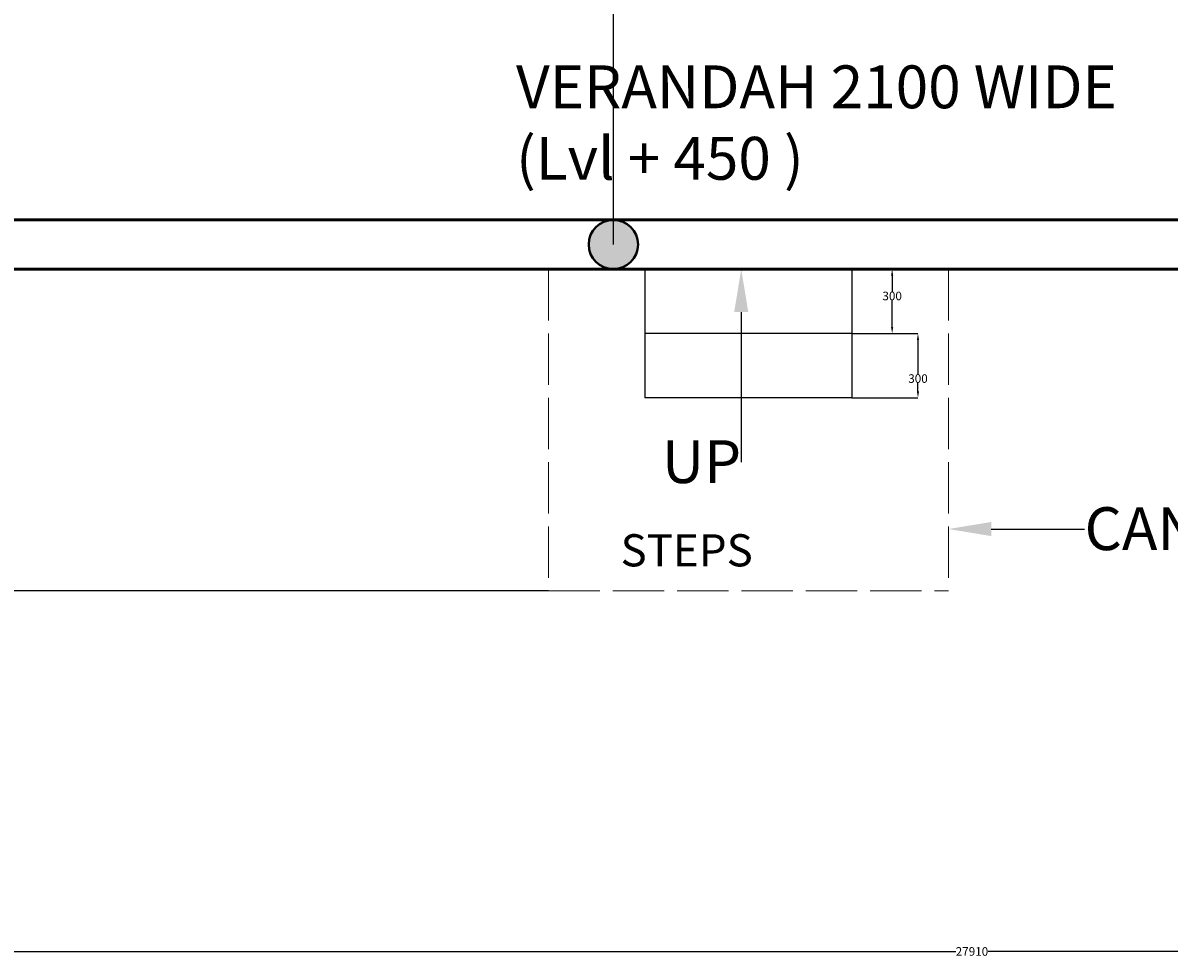
# Model space of a CAD drawing. Units: millimetres. Extents: x -17156 to 39375, y -45872 to -24892.
# Tile 4 of 12: x -5337 to 7, y -45872 to -41514. Entities that reach past the tile are written whole.
import ezdxf
from ezdxf import colors
from ezdxf.entities.mleader import LeaderData, LeaderLine
from ezdxf.math import Vec2, Vec3

# ---------------------------------------------------------------- set-up
doc = ezdxf.new("R2010")
doc.units = ezdxf.units.MM
doc.header["$MEASUREMENT"] = 0
doc.linetypes.add('ACAD_ISO02W100', pattern=[15, 12, -3])
for name, color, linetype, lineweight in [('A-ANNO-DIMS', 2, 'Continuous', 18), ('A-ANNO-TEXT', 4, 'Continuous', 18), ('A-AREA-IDEN', 4, 'Continuous', 25), ('A-COLS', 7, 'Continuous', 40), ('A-ROOF-OVHD', 8, 'ACAD_ISO02W100', 18), ('STEPS', 2, 'Continuous', 25), ('WALLS', 5, 'Continuous', 50)]:
    doc.layers.add(name, color=color, linetype=linetype, lineweight=lineweight)
doc.layers.add('A-COLS-PATT', color=114, linetype='Continuous', lineweight=13, true_color=0x139b48)
doc.styles.get("Standard").update_dxf_attribs({"font": 'arial.ttf'})
doc.dimstyles.get("Standard").update_dxf_attribs({"dimtxt": 40, "dimasz": 30.18, "dimexe": 0, "dimexo": 0.0625, "dimgap": 0.09, "dimtad": 0, "dimtih": 1, "dimtoh": 1, "dimdec": 0, "dimzin": 0, "dimdsep": 46, "dimtxsty": 'Standard', "dimcen": 0.09, "dimadec": 0, "dimazin": 0, "dimtfac": 1, "dimtdec": 0, "dimtofl": 0, "dimtmove": 0, "dimatfit": 3, "dimfxl": 1, "dimtolj": 1, "dimtzin": 0, "dimarcsym": 0})

# ---------------------------------------------------------------- blocks, each defined once
blk = doc.blocks.new('*D98')
at = {"layer": 'A-ANNO-DIMS', "color": 0, "lineweight": -2, "transparency": 16777216}
for p, q in [((-1472.3, -42962.8), (-1163.9, -42962.8)), ((-1163.9, -42993), (-1163.9, -43152.7)), ((-1163.9, -43232.7), (-1163.9, -43193.7)), ((-1472.3, -43262.8), (-1163.9, -43262.8))]:
    blk.add_line(p, q, dxfattribs=at)
at = {"layer": 'A-ANNO-DIMS', "color": 0, "lineweight": 100, "transparency": 16777216}
for points in [[(-1169, -42993), (-1158.9, -42993), (-1163.9, -42962.8)], [(-1169, -43232.7), (-1158.9, -43232.7), (-1163.9, -43262.8)]]:
    blk.add_solid(points, dxfattribs=at)
at = {"layer": 'Defpoints', "color": 0, "lineweight": 100, "transparency": 16777216}
for p in [(-1472.3, -42962.8), (-1163.9, -42962.8), (-1472.3, -43262.8)]:
    blk.add_point(p, dxfattribs=at)
at = {"layer": 'A-ANNO-DIMS', "color": 0, "transparency": 16777216, "insert": (-1163.9, -43173.2), "char_height": 40, "attachment_point": 5}
blk.add_mtext('\\A1;300', dxfattribs=at)
blk = doc.blocks.new('*D99')
at = {"layer": 'A-ANNO-DIMS', "color": 0, "lineweight": -2, "transparency": 16777216}
for p, q in [((-1472.3, -42662.8), (-1284.4, -42662.8)), ((-1284.4, -42693), (-1284.4, -42767.4)), ((-1284.4, -42932.7), (-1284.4, -42808.4)), ((-1472.3, -42962.8), (-1284.4, -42962.8))]:
    blk.add_line(p, q, dxfattribs=at)
at = {"layer": 'A-ANNO-DIMS', "color": 0, "lineweight": 100, "transparency": 16777216}
for points in [[(-1289.4, -42693), (-1279.4, -42693), (-1284.4, -42662.8)], [(-1289.4, -42932.7), (-1279.4, -42932.7), (-1284.4, -42962.8)]]:
    blk.add_solid(points, dxfattribs=at)
at = {"layer": 'Defpoints', "color": 0, "lineweight": 100, "transparency": 16777216}
for p in [(-1472.3, -42662.8), (-1284.4, -42662.8), (-1472.3, -42962.8)]:
    blk.add_point(p, dxfattribs=at)
at = {"layer": 'A-ANNO-DIMS', "color": 0, "transparency": 16777216, "insert": (-1284.4, -42787.9), "char_height": 40, "attachment_point": 5}
blk.add_mtext('\\A1;300', dxfattribs=at)
blk = doc.blocks.new('*D145')
at = {"layer": 'A-ANNO-DIMS', "color": 0, "lineweight": -2, "transparency": 16777216}
for p, q in [((-6237.4, -27247.8), (-17080.3, -27247.8)), ((-17080.3, -27278), (-17080.3, -35684.8)), ((-17080.3, -44132.7), (-17080.3, -35725.9)), ((-2887.4, -44162.8), (-17080.3, -44162.8))]:
    blk.add_line(p, q, dxfattribs=at)
at = {"layer": 'A-ANNO-DIMS', "color": 0, "lineweight": 100, "transparency": 16777216}
for points in [[(-17085.4, -27278), (-17075.3, -27278), (-17080.3, -27247.8)], [(-17085.4, -44132.7), (-17075.3, -44132.7), (-17080.3, -44162.8)]]:
    blk.add_solid(points, dxfattribs=at)
at = {"layer": 'Defpoints', "color": 0, "lineweight": 100, "transparency": 16777216}
for p in [(-6237.3, -27247.8), (-17080.3, -44162.8), (-2887.3, -44162.8)]:
    blk.add_point(p, dxfattribs=at)
at = {"layer": 'A-ANNO-DIMS', "color": 0, "transparency": 16777216, "insert": (-17080.3, -35705.3), "char_height": 40, "attachment_point": 5}
blk.add_mtext('\\A1;16915', dxfattribs=at)
blk = doc.blocks.new('*D146')
at = {"layer": 'A-ANNO-DIMS', "color": 0, "lineweight": -2, "transparency": 16777216}
for p, q in [((-14867.3, -42732.9), (-14867.3, -45845.8)), ((13042.7, -42732.9), (13042.7, -45845.8)), ((-14837.2, -45845.8), (-988, -45845.8)), ((13012.5, -45845.8), (-836.7, -45845.8))]:
    blk.add_line(p, q, dxfattribs=at)
at = {"layer": 'A-ANNO-DIMS', "color": 0, "lineweight": 100, "transparency": 16777216}
for points in [[(-14837.2, -45840.8), (-14837.2, -45850.9), (-14867.3, -45845.8)], [(13012.5, -45840.8), (13012.5, -45850.9), (13042.7, -45845.8)]]:
    blk.add_solid(points, dxfattribs=at)
at = {"layer": 'Defpoints', "color": 0, "lineweight": 100, "transparency": 16777216}
for p in [(-14867.3, -42732.8), (13042.7, -42732.8), (13042.7, -45845.8)]:
    blk.add_point(p, dxfattribs=at)
at = {"layer": 'A-ANNO-DIMS', "color": 0, "transparency": 16777216, "insert": (-912.3, -45845.8), "char_height": 40, "attachment_point": 5}
blk.add_mtext('\\A1;27910', dxfattribs=at)
blk = doc.blocks.new('*D151')
at = {"layer": 'A-ANNO-DIMS', "color": 0, "lineweight": -2, "transparency": 16777216}
for p, q in [((-6122.3, -42547.8), (-6122.3, -25564.8)), ((-6092.2, -25564.8), (-4413.2, -25564.8)), ((-2614.5, -25564.8), (-4293.5, -25564.8)), ((-2584.3, -42547.8), (-2584.3, -25564.8))]:
    blk.add_line(p, q, dxfattribs=at)
at = {"layer": 'A-ANNO-DIMS', "color": 0, "lineweight": 100, "transparency": 16777216}
for points in [[(-6092.2, -25559.8), (-6092.2, -25569.9), (-6122.3, -25564.8)], [(-2614.5, -25559.8), (-2614.5, -25569.9), (-2584.3, -25564.8)]]:
    blk.add_solid(points, dxfattribs=at)
at = {"layer": 'Defpoints', "color": 0, "lineweight": 100, "transparency": 16777216}
for p in [(-2584.3, -25564.8), (-6122.3, -42547.8), (-2584.3, -42547.8)]:
    blk.add_point(p, dxfattribs=at)
at = {"layer": 'A-ANNO-DIMS', "color": 0, "transparency": 16777216, "insert": (-4353.3, -25564.8), "char_height": 40, "attachment_point": 5}
blk.add_mtext('\\A1;3538', dxfattribs=at)

msp = doc.modelspace()

# ---------------------------------------------------------------- hatches: boundary and pattern name
at = {"layer": 'A-COLS-PATT'}
h = msp.add_hatch(color=256, dxfattribs=at)
h.dxf.hatch_style = 1
h.paths.add_polyline_path([(-6007.35, -42547.85, 1), (-6237.35, -42547.85, 1)])
h.paths.add_polyline_path([(-2699.35, -42547.85, 1), (-2469.35, -42547.85, 1)])
h.paths.add_polyline_path([(424.65, -42547.85, 1), (654.65, -42547.85, 1)])
h.paths.add_polyline_path([(3997.65, -42547.85, 1), (4227.65, -42547.85, 1)])
h.paths.add_polyline_path([(1581.84, -34499.85), (1481.84, -34499.85), (1481.84, -34599.85), (1581.84, -34599.85)])
h.paths.add_polyline_path([(3181.84, -34499.85), (3081.84, -34499.85), (3081.84, -34599.85), (3181.84, -34599.85)])
h.paths.add_polyline_path([(-162.32, -34499.85), (-262.32, -34499.85), (-262.32, -34599.85), (-162.32, -34599.85)])
h.paths.add_polyline_path([(-1762.32, -34499.85), (-1862.32, -34499.85), (-1862.32, -34599.85), (-1762.32, -34599.85)])
h.paths.add_polyline_path([(-3445.85, -34499.85), (-3545.85, -34499.85), (-3545.85, -34599.85), (-3445.85, -34599.85)])
h.paths.add_polyline_path([(-5045.85, -34499.85), (-5145.85, -34499.85), (-5145.85, -34599.85), (-5045.85, -34599.85)])

# ---------------------------------------------------------------- linework, layer by layer
at = {"layer": 'A-COLS'}
msp.add_circle((-2584.35, -42547.85), 115, dxfattribs=at)
at = {"layer": 'A-ROOF-OVHD', "ltscale": 20}
for p, q in [((-2887.35, -42662.85), (-2887.35, -44162.85)), ((-1022.35, -42662.85), (-1022.35, -44162.85)), ((-2887.35, -44162.85), (-1022.35, -44162.85))]:
    msp.add_line(p, q, dxfattribs=at)
at = {"layer": 'STEPS'}
for p, q in [((-2437.35, -42662.85), (-2437.35, -43262.85)), ((-1472.35, -42662.85), (-1472.35, -43262.85)), ((-1472.35, -42962.85), (-2437.35, -42962.85)), ((-1472.35, -43262.85), (-2437.35, -43262.85))]:
    msp.add_line(p, q, dxfattribs=at)
at = {"layer": 'WALLS'}
for p, q in [((12592.65, -42432.85), (-10997.35, -42432.85)), ((12822.65, -42662.85), (-14797.35, -42662.85))]:
    msp.add_line(p, q, dxfattribs=at)

# ---------------------------------------------------------------- texts
at = {"layer": 'A-ANNO-TEXT', "insert": (-2550.74, -43899.35), "char_height": 150, "attachment_point": 1}
msp.add_mtext_dynamic_manual_height_columns('{STEPS}', width=605.9062, gutter_width=1, heights=[0], dxfattribs=at)
at = {"layer": 'A-AREA-IDEN', "insert": (-3038.04, -41712.25), "char_height": 200, "attachment_point": 1}
msp.add_mtext_dynamic_manual_height_columns('{VERANDAH 2100 WIDE\\P(Lvl + 450 )}', width=5045.4894, gutter_width=1, heights=[0], dxfattribs=at)

# ---------------------------------------------------------------- dimensions: what is measured, and where the dimension line sits
at = {"layer": 'A-ANNO-DIMS'}
for base, p1, p2, picture, middle in [((-2584.35, -25564.85), (-6122.35, -42547.85), (-2584.35, -42547.85), '*D151', (-4353.35, -25564.85)), ((13042.65, -45845.85), (-14867.35, -42732.85), (13042.65, -42732.85), '*D146', (-912.35, -45845.85))]:
    dim = msp.add_linear_dim(base=base, p1=p1, p2=p2, dimstyle='Standard', override={"dimdec": 0, "dimlfac": 1, "dimrnd": 0, "dimzin": 0, "dimdsep": 46, "dimlunit": 2}, dxfattribs=at)
    dim.commit()
    dim.dimension.update_dxf_attribs({"geometry": picture, "text_midpoint": middle})
dim = msp.add_linear_dim(base=(-17080.35, -44162.85), p1=(-6237.35, -27247.85), p2=(-2887.35, -44162.85), angle=90, dimstyle='Standard', override={"dimdec": 0, "dimlfac": 1, "dimrnd": 0, "dimzin": 0, "dimdsep": 46, "dimlunit": 2}, dxfattribs=at)
dim.commit()
dim.dimension.update_dxf_attribs({"geometry": '*D145', "text_midpoint": (-17080.35, -35705.35)})
for base, p1, p2, picture, middle in [((-1284.39, -42662.85), (-1472.35, -42962.85), (-1472.35, -42662.85), '*D99', (-1284.39, -42787.91)), ((-1163.92, -42962.85), (-1472.35, -43262.85), (-1472.35, -42962.85), '*D98', (-1163.92, -43173.21))]:
    dim = msp.add_linear_dim(base=base, p1=p1, p2=p2, angle=270, dimstyle='Standard', override={"dimclrd": 0, "dimclre": 0, "dimclrt": 0}, dxfattribs=at)
    dim.commit()
    dim.dimension.update_dxf_attribs({"geometry": picture, "text_midpoint": middle, "dimtype": 160})

# ---------------------------------------------------------------- leaders
at = {"layer": 'A-ANNO-TEXT'}
ml = msp.add_multileader_mtext('Standard', dxfattribs=at)
ml.set_content('{\\C4;UP}', color=256)
ml.set_leader_properties()
ml.build(insert=Vec2(0, 0))
ml.multileader.update_dxf_attribs({"dogleg_length": 0.36, "arrow_head_size": 200})
ctx = ml.context
ctx.base_point, ctx.char_height, ctx.arrow_head_size, ctx.landing_gap_size, ctx.plane_origin = Vec3(-2342.61, -43562.47), 200, 200, 0.09, Vec3(-1988.04, -42662.85)
ctx.text_align_type = 2
notes = []
notes.append((ctx, [(0, (1, 1, 0), (-1988.04, -43562.47), (-1, 0), 0.36, [(0, [(-1988.04, -42662.85)], 0, [])])]))
ctx.mtext.insert, ctx.mtext.alignment, ctx.mtext.flow_direction = Vec3(-1988.49, -43460.76), 3, 5
ml = msp.add_multileader_mtext('Standard', dxfattribs=at)
ml.set_content('{\\C4;CANOPY}', color=256)
ml.set_leader_properties()
ml.build(insert=Vec2(0, 0))
ml.multileader.update_dxf_attribs({"dogleg_length": 0.36, "arrow_head_size": 200})
ctx = ml.context
ctx.base_point, ctx.char_height, ctx.arrow_head_size, ctx.landing_gap_size, ctx.plane_origin = Vec3(-387.3, -43875.13), 200, 200, 0.09, Vec3(-1022.35, -43875.13)
notes.append((ctx, [(0, (1, 1, 0), (-387.66, -43875.13), (1, 0), 0.36, [(0, [(-1022.35, -43875.13)], 0, [])])]))
ctx.mtext.insert, ctx.mtext.flow_direction = Vec3(-387.21, -43773.42), 5
for ctx, leaders in notes:
    for number, flags, end, landing, length, lines in leaders:
        leader = LeaderData()
        leader.index, (leader.has_last_leader_line, leader.has_dogleg_vector, leader.attachment_direction) = number, flags
        leader.last_leader_point, leader.dogleg_vector, leader.dogleg_length = Vec3(end), Vec3(landing), length
        for number, points, colour, breaks in lines:
            line = LeaderLine()
            line.index, line.vertices, line.color, line.breaks = number, Vec3.list(points), colors.encode_raw_color(colour), breaks
            leader.lines.append(line)
        ctx.leaders.append(leader)

doc.saveas('drawing.dxf')
